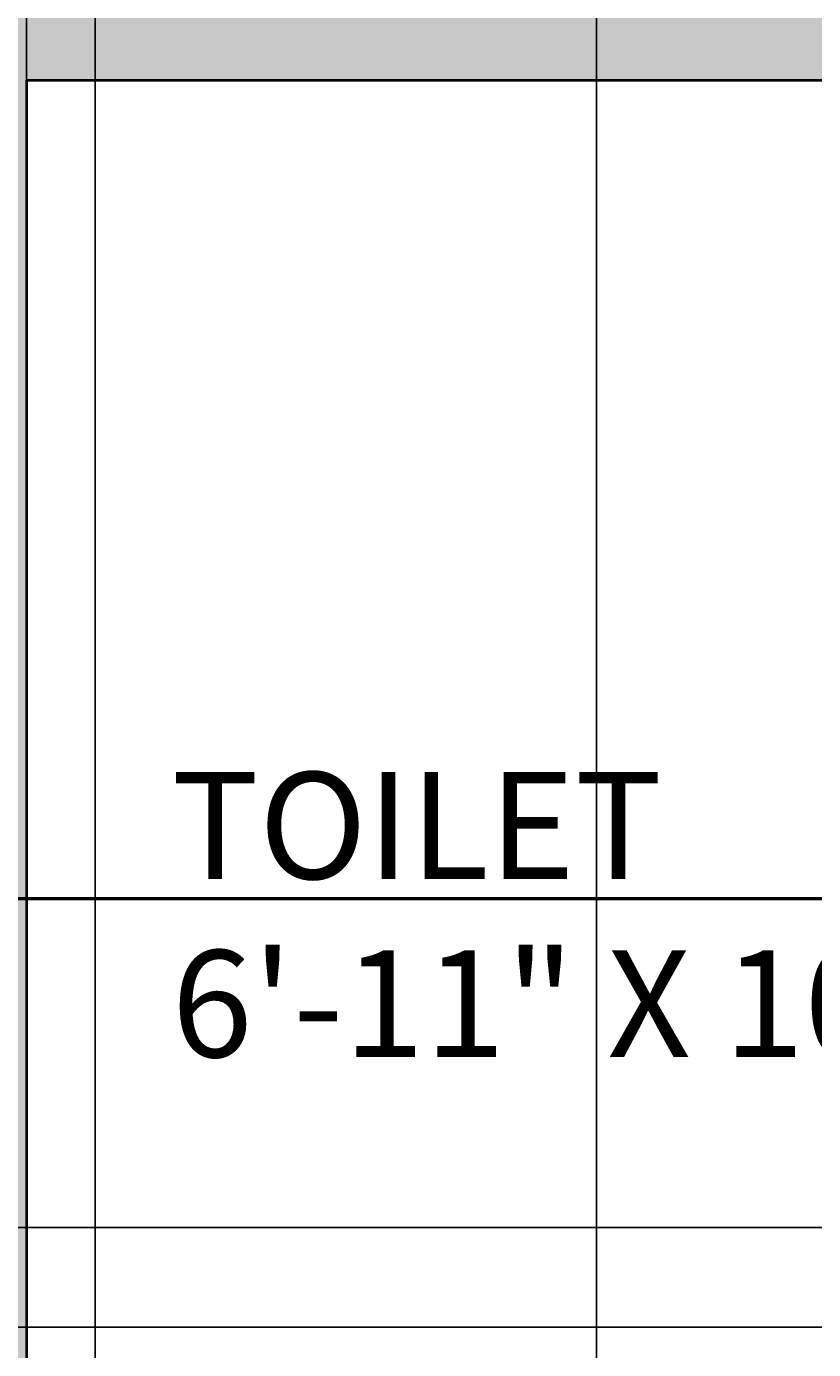
# Model space of a CAD drawing. Units: inches. Extents: x 818 to 1898, y 976 to 2364.
# Tile 45 of 96: x 1623 to 1667, y 1520 to 1594. Entities that reach past the tile are written whole.
import ezdxf

# ---------------------------------------------------------------- set-up
doc = ezdxf.new("R2010")
doc.units = ezdxf.units.IN
doc.header["$LTSCALE"] = 5
doc.header["$MEASUREMENT"] = 0
for name, color, linetype, lineweight in [('A-ANNO-DIMS', 2, 'Continuous', 18), ('A-AREA-IDEN', 7, 'Continuous', 18), ('A-WALL', 7, 'Continuous', 40)]:
    doc.layers.add(name, color=color, linetype=linetype, lineweight=lineweight)
doc.layers.add('A-WALL-PATT', color=251, linetype='Continuous', lineweight=13, true_color=0x636466)
doc.styles.get("Standard").update_dxf_attribs({"font": 'arial.ttf'})
doc.dimstyles.get("Standard").update_dxf_attribs({"dimtxt": 0.18, "dimasz": 0.18, "dimexe": 0.18, "dimexo": 0.0625, "dimgap": 0.09, "dimtad": 0, "dimtih": 1, "dimtoh": 1, "dimdec": 4, "dimzin": 0, "dimdsep": 46, "dimtxsty": 'Standard', "dimcen": 0.09, "dimadec": 0, "dimazin": 0, "dimtfac": 1, "dimtdec": 4, "dimtofl": 0, "dimtmove": 0, "dimatfit": 3, "dimfxl": 1, "dimtolj": 1, "dimtzin": 0, "dimarcsym": 0})

# ---------------------------------------------------------------- blocks, each defined once
blk = doc.blocks.new('*D102')
at = {"layer": 'A-ANNO-DIMS', "color": 0, "lineweight": -2, "ltscale": 5, "transparency": 16777216}
for p, q in [((1565.483, 1071.118), (1565.483, 2363.873)), ((1565.663, 2363.693), (1595.635, 2363.693)), ((1626.395, 2363.693), (1596.423, 2363.693)), ((1626.575, 1071.118), (1626.575, 2363.873))]:
    blk.add_line(p, q, dxfattribs=at)
at = {"layer": 'A-ANNO-DIMS', "color": 0, "ltscale": 5, "transparency": 16777216}
for points in [[(1565.663, 2363.723), (1565.663, 2363.663), (1565.483, 2363.693)], [(1626.395, 2363.723), (1626.395, 2363.663), (1626.575, 2363.693)]]:
    blk.add_solid(points, dxfattribs=at)
at = {"layer": 'Defpoints', "color": 0, "ltscale": 5, "transparency": 16777216}
for p in [(1626.575, 2363.693), (1565.483, 1071.055), (1626.575, 1071.055)]:
    blk.add_point(p, dxfattribs=at)
at = {"layer": 'A-ANNO-DIMS', "color": 0, "ltscale": 5, "transparency": 16777216, "insert": (1596.029, 2363.693), "char_height": 0.18, "attachment_point": 5}
blk.add_mtext('\\A1;61.09', dxfattribs=at)
blk = doc.blocks.new('*D103')
at = {"layer": 'A-ANNO-DIMS', "color": 0, "lineweight": -2, "ltscale": 5, "transparency": 16777216}
for p, q in [((1626.575, 1071.118), (1626.575, 2363.873)), ((1626.755, 2363.693), (1657.699, 2363.693)), ((1689.291, 2363.693), (1658.348, 2363.693)), ((1689.471, 1071.118), (1689.471, 2363.873))]:
    blk.add_line(p, q, dxfattribs=at)
at = {"layer": 'A-ANNO-DIMS', "color": 0, "ltscale": 5, "transparency": 16777216}
for points in [[(1626.755, 2363.723), (1626.755, 2363.663), (1626.575, 2363.693)], [(1689.291, 2363.723), (1689.291, 2363.663), (1689.471, 2363.693)]]:
    blk.add_solid(points, dxfattribs=at)
at = {"layer": 'Defpoints', "color": 0, "ltscale": 5, "transparency": 16777216}
for p in [(1689.471, 2363.693), (1626.575, 1071.055), (1689.471, 1071.055)]:
    blk.add_point(p, dxfattribs=at)
at = {"layer": 'A-ANNO-DIMS', "color": 0, "ltscale": 5, "transparency": 16777216, "insert": (1658.023, 2363.693), "char_height": 0.18, "attachment_point": 5}
blk.add_mtext('\\A1;62.9', dxfattribs=at)
blk = doc.blocks.new('*D117')
at = {"layer": 'A-ANNO-DIMS', "color": 0, "lineweight": -2, "ltscale": 5, "transparency": 16777216}
for p, q in [((1766.29, 1545.183), (818.026, 1545.183)), ((818.206, 1545.003), (818.206, 1501.178)), ((818.206, 1456.989), (818.206, 1500.814)), ((1766.29, 1456.809), (818.026, 1456.809))]:
    blk.add_line(p, q, dxfattribs=at)
at = {"layer": 'A-ANNO-DIMS', "color": 0, "ltscale": 5, "transparency": 16777216}
for points in [[(818.176, 1545.003), (818.236, 1545.003), (818.206, 1545.183)], [(818.176, 1456.989), (818.236, 1456.989), (818.206, 1456.809)]]:
    blk.add_solid(points, dxfattribs=at)
at = {"layer": 'Defpoints', "color": 0, "ltscale": 5, "transparency": 16777216}
for p in [(818.206, 1545.183), (1766.352, 1545.183), (1766.352, 1456.809)]:
    blk.add_point(p, dxfattribs=at)
at = {"layer": 'A-ANNO-DIMS', "color": 0, "ltscale": 5, "transparency": 16777216, "insert": (818.206, 1500.996), "char_height": 0.18, "attachment_point": 5}
blk.add_mtext('\\A1;88.37', dxfattribs=at)
blk = doc.blocks.new('*D118')
at = {"layer": 'A-ANNO-DIMS', "color": 0, "lineweight": -2, "ltscale": 5, "transparency": 16777216}
for p, q in [((1766.29, 1627.505), (818.026, 1627.505)), ((818.206, 1627.325), (818.206, 1586.526)), ((818.206, 1545.363), (818.206, 1586.162)), ((1766.29, 1545.183), (818.026, 1545.183))]:
    blk.add_line(p, q, dxfattribs=at)
at = {"layer": 'A-ANNO-DIMS', "color": 0, "ltscale": 5, "transparency": 16777216}
for points in [[(818.176, 1627.325), (818.236, 1627.325), (818.206, 1627.505)], [(818.176, 1545.363), (818.236, 1545.363), (818.206, 1545.183)]]:
    blk.add_solid(points, dxfattribs=at)
at = {"layer": 'Defpoints', "color": 0, "ltscale": 5, "transparency": 16777216}
for p in [(818.206, 1627.505), (1766.352, 1627.505), (1766.352, 1545.183)]:
    blk.add_point(p, dxfattribs=at)
at = {"layer": 'A-ANNO-DIMS', "color": 0, "ltscale": 5, "transparency": 16777216, "insert": (818.206, 1586.344), "char_height": 0.18, "attachment_point": 5}
blk.add_mtext('\\A1;82.32', dxfattribs=at)
blk = doc.blocks.new('*D170')
at = {"layer": 'A-ANNO-DIMS', "color": 0, "lineweight": -2, "ltscale": 5, "transparency": 16777216}
for p, q in [((1430.788, 1600.078), (1897.916, 1600.078)), ((1897.736, 1599.898), (1897.736, 1550.76)), ((1897.736, 1501.258), (1897.736, 1550.396)), ((1430.788, 1501.078), (1897.916, 1501.078))]:
    blk.add_line(p, q, dxfattribs=at)
at = {"layer": 'A-ANNO-DIMS', "color": 0, "ltscale": 5, "transparency": 16777216}
for points in [[(1897.706, 1599.898), (1897.766, 1599.898), (1897.736, 1600.078)], [(1897.706, 1501.258), (1897.766, 1501.258), (1897.736, 1501.078)]]:
    blk.add_solid(points, dxfattribs=at)
at = {"layer": 'Defpoints', "color": 0, "ltscale": 5, "transparency": 16777216}
for p in [(1430.725, 1600.078), (1897.736, 1600.078), (1430.725, 1501.078)]:
    blk.add_point(p, dxfattribs=at)
at = {"layer": 'A-ANNO-DIMS', "color": 0, "ltscale": 5, "transparency": 16777216, "insert": (1897.736, 1550.578), "char_height": 0.18, "attachment_point": 5}
blk.add_mtext('\\A1;99', dxfattribs=at)
blk = doc.blocks.new('*D173')
at = {"layer": 'A-ANNO-DIMS', "color": 0, "lineweight": -2, "ltscale": 5, "transparency": 16777216}
for p, q in [((1622.725, 1463.141), (1622.725, 2363.873)), ((1622.905, 2363.693), (1638.507, 2363.693)), ((1654.545, 2363.693), (1638.943, 2363.693)), ((1654.725, 1463.141), (1654.725, 2363.873))]:
    blk.add_line(p, q, dxfattribs=at)
at = {"layer": 'A-ANNO-DIMS', "color": 0, "ltscale": 5, "transparency": 16777216}
for points in [[(1622.905, 2363.723), (1622.905, 2363.663), (1622.725, 2363.693)], [(1654.545, 2363.723), (1654.545, 2363.663), (1654.725, 2363.693)]]:
    blk.add_solid(points, dxfattribs=at)
at = {"layer": 'Defpoints', "color": 0, "ltscale": 5, "transparency": 16777216}
for p in [(1654.725, 2363.693), (1622.725, 1463.078), (1654.725, 1463.078)]:
    blk.add_point(p, dxfattribs=at)
at = {"layer": 'A-ANNO-DIMS', "color": 0, "ltscale": 5, "transparency": 16777216, "insert": (1638.725, 2363.693), "char_height": 0.18, "attachment_point": 5}
blk.add_mtext('\\A1;32', dxfattribs=at)
blk = doc.blocks.new('*D180')
at = {"layer": 'A-ANNO-DIMS', "color": 0, "lineweight": -2, "ltscale": 5, "transparency": 16777216}
for p, q in [((1599.725, 1639.516), (1599.725, 975.663)), ((1669.725, 1639.516), (1669.725, 975.663)), ((1599.905, 975.843), (1634.507, 975.843)), ((1669.545, 975.843), (1634.943, 975.843))]:
    blk.add_line(p, q, dxfattribs=at)
at = {"layer": 'A-ANNO-DIMS', "color": 0, "ltscale": 5, "transparency": 16777216}
for points in [[(1599.905, 975.873), (1599.905, 975.813), (1599.725, 975.843)], [(1669.545, 975.873), (1669.545, 975.813), (1669.725, 975.843)]]:
    blk.add_solid(points, dxfattribs=at)
at = {"layer": 'Defpoints', "color": 0, "ltscale": 5, "transparency": 16777216}
for p in [(1599.725, 1639.578), (1669.725, 1639.578), (1669.725, 975.843)]:
    blk.add_point(p, dxfattribs=at)
at = {"layer": 'A-ANNO-DIMS', "color": 0, "ltscale": 5, "transparency": 16777216, "insert": (1634.725, 975.843), "char_height": 0.18, "attachment_point": 5}
blk.add_mtext('\\A1;70', dxfattribs=at)
blk = doc.blocks.new('*D187')
at = {"layer": 'A-ANNO-DIMS', "color": 0, "lineweight": -2, "ltscale": 5, "transparency": 16777216}
for p, q in [((1705.663, 1545.078), (818.026, 1545.078)), ((818.206, 1544.898), (818.206, 1533.259)), ((818.206, 1521.258), (818.206, 1532.898)), ((1705.663, 1521.078), (818.026, 1521.078))]:
    blk.add_line(p, q, dxfattribs=at)
at = {"layer": 'A-ANNO-DIMS', "color": 0, "ltscale": 5, "transparency": 16777216}
for points in [[(818.176, 1544.898), (818.236, 1544.898), (818.206, 1545.078)], [(818.176, 1521.258), (818.236, 1521.258), (818.206, 1521.078)]]:
    blk.add_solid(points, dxfattribs=at)
at = {"layer": 'Defpoints', "color": 0, "ltscale": 5, "transparency": 16777216}
for p in [(818.206, 1545.078), (1705.725, 1545.078), (1705.725, 1521.078)]:
    blk.add_point(p, dxfattribs=at)
at = {"layer": 'A-ANNO-DIMS', "color": 0, "ltscale": 5, "transparency": 16777216, "insert": (818.206, 1533.078), "char_height": 0.18, "attachment_point": 5}
blk.add_mtext('\\A1;24', dxfattribs=at)
blk = doc.blocks.new('*D197')
at = {"layer": 'A-ANNO-DIMS', "color": 0, "lineweight": -2, "ltscale": 5, "transparency": 16777216}
for p, q in [((1457.788, 1526.671), (1897.916, 1526.671)), ((1897.736, 1526.491), (1897.736, 1468.076)), ((1897.736, 1409.298), (1897.736, 1467.713)), ((1457.788, 1409.118), (1897.916, 1409.118))]:
    blk.add_line(p, q, dxfattribs=at)
at = {"layer": 'A-ANNO-DIMS', "color": 0, "ltscale": 5, "transparency": 16777216}
for points in [[(1897.706, 1526.491), (1897.766, 1526.491), (1897.736, 1526.671)], [(1897.706, 1409.298), (1897.766, 1409.298), (1897.736, 1409.118)]]:
    blk.add_solid(points, dxfattribs=at)
at = {"layer": 'Defpoints', "color": 0, "ltscale": 5, "transparency": 16777216}
for p in [(1457.725, 1526.671), (1897.736, 1526.671), (1457.725, 1409.118)]:
    blk.add_point(p, dxfattribs=at)
at = {"layer": 'A-ANNO-DIMS', "color": 0, "ltscale": 5, "transparency": 16777216, "insert": (1897.736, 1467.894), "char_height": 0.18, "attachment_point": 5}
blk.add_mtext('\\A1;117.55', dxfattribs=at)
blk = doc.blocks.new('*D198')
at = {"layer": 'A-ANNO-DIMS', "color": 0, "lineweight": -2, "ltscale": 5, "transparency": 16777216}
for p, q in [((1741.841, 1545.016), (1741.841, 975.663)), ((1430.725, 1346.016), (1430.725, 975.663)), ((1430.905, 975.843), (1585.907, 975.843)), ((1741.661, 975.843), (1586.659, 975.843))]:
    blk.add_line(p, q, dxfattribs=at)
at = {"layer": 'A-ANNO-DIMS', "color": 0, "ltscale": 5, "transparency": 16777216}
for points in [[(1430.905, 975.873), (1430.905, 975.813), (1430.725, 975.843)], [(1741.661, 975.873), (1741.661, 975.813), (1741.841, 975.843)]]:
    blk.add_solid(points, dxfattribs=at)
at = {"layer": 'Defpoints', "color": 0, "ltscale": 5, "transparency": 16777216}
for p in [(1741.841, 1545.078), (1430.725, 1346.078), (1741.841, 975.843)]:
    blk.add_point(p, dxfattribs=at)
at = {"layer": 'A-ANNO-DIMS', "color": 0, "ltscale": 5, "transparency": 16777216, "insert": (1586.283, 975.843), "char_height": 0.18, "attachment_point": 5}
blk.add_mtext('\\A1;311.1', dxfattribs=at)
blk = doc.blocks.new('*D199')
at = {"layer": 'A-ANNO-DIMS', "color": 0, "lineweight": -2, "ltscale": 5, "transparency": 16777216}
for p, q in [((1559.788, 1687.078), (1897.916, 1687.078)), ((1897.736, 1686.898), (1897.736, 1513.154)), ((1897.736, 1339.045), (1897.736, 1512.79)), ((1660.377, 1338.865), (1897.916, 1338.865))]:
    blk.add_line(p, q, dxfattribs=at)
at = {"layer": 'A-ANNO-DIMS', "color": 0, "ltscale": 5, "transparency": 16777216}
for points in [[(1897.706, 1686.898), (1897.766, 1686.898), (1897.736, 1687.078)], [(1897.706, 1339.045), (1897.766, 1339.045), (1897.736, 1338.865)]]:
    blk.add_solid(points, dxfattribs=at)
at = {"layer": 'Defpoints', "color": 0, "ltscale": 5, "transparency": 16777216}
for p in [(1559.725, 1687.078), (1897.736, 1687.078), (1660.314, 1338.865)]:
    blk.add_point(p, dxfattribs=at)
at = {"layer": 'A-ANNO-DIMS', "color": 0, "ltscale": 5, "transparency": 16777216, "insert": (1897.736, 1512.972), "char_height": 0.18, "attachment_point": 5}
blk.add_mtext('\\A1;348.2', dxfattribs=at)
blk = doc.blocks.new('*D214')
at = {"layer": 'A-ANNO-DIMS', "color": 0, "lineweight": -2, "ltscale": 5, "transparency": 16777216}
for p, q in [((1511.725, 1687.016), (1511.725, 975.663)), ((1714.725, 1687.016), (1714.725, 975.663)), ((1511.905, 975.843), (1612.935, 975.843)), ((1714.545, 975.843), (1613.516, 975.843))]:
    blk.add_line(p, q, dxfattribs=at)
at = {"layer": 'A-ANNO-DIMS', "color": 0, "ltscale": 5, "transparency": 16777216}
for points in [[(1511.905, 975.873), (1511.905, 975.813), (1511.725, 975.843)], [(1714.545, 975.873), (1714.545, 975.813), (1714.725, 975.843)]]:
    blk.add_solid(points, dxfattribs=at)
at = {"layer": 'Defpoints', "color": 0, "ltscale": 5, "transparency": 16777216}
for p in [(1511.725, 1687.078), (1714.725, 1687.078), (1714.725, 975.843)]:
    blk.add_point(p, dxfattribs=at)
at = {"layer": 'A-ANNO-DIMS', "color": 0, "ltscale": 5, "transparency": 16777216, "insert": (1613.225, 975.843), "char_height": 0.18, "attachment_point": 5}
blk.add_mtext('\\A1;203', dxfattribs=at)

msp = doc.modelspace()

# ---------------------------------------------------------------- hatches: boundary and pattern name
at = {"layer": 'A-WALL-PATT', "ltscale": 5}
h = msp.add_hatch(color=256, dxfattribs=at)
h.dxf.hatch_style = 1
h.paths.add_polyline_path([(1267.7252, 1928.9218), (1258.7252, 1928.9218), (1258.7252, 1913.6401), (1250.3029, 1913.6401), (1250.3029, 1878.3919), (1258.7252, 1878.3919), (1258.7252, 1862.9652), (1267.7252, 1862.9652)])
h.paths.add_polyline_path([(1267.7252, 1814.9652), (1258.7252, 1814.9652), (1258.7252, 1755.3321), (1267.7252, 1755.3321)])
h.paths.add_polyline_path([(1463.7252, 1696.0782), (1267.7252, 1696.0782), (1267.7252, 1707.3321), (1258.7252, 1707.3321), (1258.7252, 1700.0782), (1251.9333, 1700.0782), (1251.9333, 1687.0782), (1463.7252, 1687.0782)])
h.paths.add_polyline_path([(1714.7251, 1717.3178), (1705.7251, 1717.3178), (1705.7251, 1696.0782), (1599.7251, 1696.0782), (1599.7251, 1790.0782), (1705.7251, 1790.0782), (1705.7251, 1785.6125), (1714.7251, 1785.6125), (1714.7251, 1827.2125), (1705.7251, 1827.2125), (1705.7251, 1802.0782), (1599.7251, 1802.0782), (1599.7251, 1867.0782), (1705.7251, 1867.0782), (1705.7251, 1857.2125), (1714.7251, 1857.2125), (1714.7251, 1930.0316), (1741.8409, 1930.0316), (1741.8409, 1935.0316), (1714.7251, 1935.0316), (1714.7251, 1957.0338), (1741.8409, 1957.0338), (1741.8409, 1962.0338), (1714.7251, 1962.0338), (1705.7251, 1962.0338), (1705.7251, 1948.0782), (1599.7251, 1948.0782), (1599.7251, 1981.0782), (1590.7252, 1981.0782), (1590.7252, 1941.0782), (1620.7252, 1941.0782), (1705.7251, 1941.0782), (1705.7251, 1876.0782), (1599.7251, 1876.0782), (1599.7251, 1911.0782), (1590.7252, 1911.0782), (1590.7252, 1876.0782), (1429.2252, 1876.0782), (1429.2252, 1867.0782), (1511.7251, 1867.0782), (1528.593, 1867.0782), (1595.7252, 1867.0782), (1595.7252, 1773.0782), (1520.7252, 1773.0782), (1520.7252, 1837.5823), (1532.593, 1837.5823), (1532.593, 1867.0782), (1528.593, 1867.0782), (1528.593, 1841.5823), (1511.7251, 1841.5823), (1511.7251, 1744.9714), (1520.7252, 1744.9714), (1520.7252, 1761.0782), (1595.7252, 1761.0782), (1595.7252, 1696.0782), (1520.7252, 1696.0782), (1520.7252, 1716.0454), (1511.7251, 1716.0454), (1511.7251, 1696.0782), (1511.7251, 1687.0782), (1714.7251, 1687.0782)])
h.paths.add_polyline_path([(1714.7251, 2053.0782), (1714.7251, 2081.1881), (1709.7252, 2081.1881), (1709.7252, 2053.0782), (1681.6446, 2053.0782), (1681.6446, 2081.1881), (1676.6446, 2081.1881), (1676.6446, 2053.0782), (1538.5155, 2053.0782), (1538.5155, 2044.0782), (1590.7252, 2044.0782), (1590.7252, 2011.0782), (1599.7251, 2011.0782), (1599.7251, 2044.0782), (1705.7251, 2044.0782), (1705.7251, 2014.5114), (1714.7251, 2014.5114)])
h.paths.add_polyline_path([(1485.1216, 2053.0782), (1422.02, 2053.0782), (1422.02, 2081.1881), (1413.02, 2081.1881), (1413.02, 2053.0782), (1399.6356, 2053.0782), (1399.6356, 2081.1881), (1390.6356, 2081.1881), (1390.6356, 2053.0782), (1388.0315, 2053.0782), (1388.0315, 2044.0782), (1416.2743, 2044.0782), (1485.1216, 2044.0782)])
h.paths.add_polyline_path([(1330.305, 2053.0782), (1258.7252, 2053.0782), (1258.7252, 2019.2871), (1267.7252, 2019.2871), (1267.7252, 2044.0782), (1330.305, 2044.0782)])
h.paths.add_polyline_path([(1258.7252, 2053.0782), (1214.6577, 2053.0782), (1214.6577, 2044.0782), (1258.7252, 2044.0782)])
h.paths.add_polyline_path([(1214.6577, 2053.0782), (1180.349, 2053.0782), (1180.349, 2044.0782), (1214.6577, 2044.0782)])
h.paths.add_polyline_path([(1714.7251, 1639.5782), (1741.8409, 1639.5782), (1741.8409, 1643.5782), (1714.7251, 1643.5782), (1714.7251, 1649.9029), (1705.7251, 1649.9029), (1705.7251, 1600.0782), (1477.7252, 1600.0782), (1477.7252, 1591.0782), (1520.7252, 1591.0782), (1616.7252, 1591.0782), (1616.7252, 1416.6857), (1622.7251, 1416.6857), (1622.7251, 1463.0782), (1624.7252, 1463.0782), (1624.7252, 1467.0782), (1622.7251, 1467.0782), (1622.7251, 1591.0782), (1705.7251, 1591.0782), (1705.7251, 1545.0782), (1714.7251, 1545.0782), (1741.8409, 1545.0782), (1741.8409, 1549.0782), (1714.7251, 1549.0782), (1714.7251, 1593.9175), (1737.8409, 1593.9175), (1737.8409, 1597.9175), (1714.7251, 1597.9175)])
h.paths.add_polyline_path([(1674.9024, 2060.7419), (1714.7045, 2060.7419), (1714.7045, 2073.1061), (1674.9024, 2073.1061)], flags=25)
h.paths.add_polyline_path([(1394.5468, 2061.6618), (1422.2344, 2061.6618), (1422.2344, 2074.0261), (1394.5468, 2074.0261)], flags=24)

# ---------------------------------------------------------------- linework, layer by layer
at = {"layer": 'A-WALL'}
for q in [(1622.7251, 1467.0782), (1705.7251, 1591.0782)]:
    msp.add_line((1622.7251, 1591.0782), q, dxfattribs=at)

# ---------------------------------------------------------------- texts
at = {"layer": 'A-AREA-IDEN', "ltscale": 5, "insert": (1630.8716, 1552.2375), "char_height": 6, "attachment_point": 1}
msp.add_mtext_dynamic_manual_height_columns('TOILET\\P6\'-11" X 10\'-4"', width=118.992422, gutter_width=1, heights=[0], dxfattribs=at)

# ---------------------------------------------------------------- dimensions: what is measured, and where the dimension line sits
at = {"layer": 'A-ANNO-DIMS', "ltscale": 5}
for base, p1, p2, override, picture, middle in [((1626.5748, 2363.6929), (1565.4835, 1071.0552), (1626.5748, 1071.0552), {"dimdec": 2, "dimlfac": 1, "dimrnd": 0, "dimzin": 0, "dimdsep": 46, "dimlunit": 2}, '*D102', (1596.0291, 2363.6929)), ((1654.7251, 2363.6929), (1622.7251, 1463.0782), (1654.7251, 1463.0782), {"dimdec": 0, "dimlfac": 1, "dimrnd": 0, "dimzin": 0, "dimdsep": 46, "dimlunit": 2}, '*D173', (1638.7251, 2363.6929)), ((1689.4714, 2363.6929), (1626.5748, 1071.0552), (1689.4714, 1071.0552), {"dimdec": 1, "dimlfac": 1, "dimrnd": 0, "dimzin": 0, "dimdsep": 46, "dimlunit": 2}, '*D103', (1658.0231, 2363.6929)), ((1714.7251, 975.8433), (1511.7251, 1687.0782), (1714.7251, 1687.0782), {"dimdec": 0, "dimlfac": 1, "dimrnd": 0, "dimzin": 0, "dimdsep": 46, "dimlunit": 2}, '*D214', (1613.2251, 975.8433)), ((1669.7251, 975.8433), (1599.7251, 1639.5782), (1669.7251, 1639.5782), {"dimdec": 0, "dimlfac": 1, "dimrnd": 0, "dimzin": 0, "dimdsep": 46, "dimlunit": 2}, '*D180', (1634.7251, 975.8433)), ((1741.8409, 975.8433), (1430.7251, 1346.0782), (1741.8409, 1545.0782), {"dimdec": 1, "dimlfac": 1, "dimrnd": 0, "dimzin": 0, "dimdsep": 46, "dimlunit": 2}, '*D198', (1586.283, 975.8433))]:
    dim = msp.add_linear_dim(base=base, p1=p1, p2=p2, dimstyle='Standard', override=override, dxfattribs=at)
    dim.commit()
    dim.dimension.update_dxf_attribs({"geometry": picture, "text_midpoint": middle})
for base, p1, p2, override, picture, middle in [((1897.736, 1687.0782), (1660.3141, 1338.8654), (1559.7251, 1687.0782), {"dimdec": 1, "dimlfac": 1, "dimrnd": 0, "dimzin": 0, "dimdsep": 46, "dimlunit": 2}, '*D199', (1897.736, 1512.9718)), ((818.2059, 1627.5052), (1766.3524, 1545.1827), (1766.3524, 1627.5052), {"dimdec": 2, "dimlfac": 1, "dimrnd": 0, "dimzin": 0, "dimdsep": 46, "dimlunit": 2}, '*D118', (818.2059, 1586.3439)), ((1897.736, 1600.0782), (1430.7251, 1501.0782), (1430.7251, 1600.0782), {"dimdec": 0, "dimlfac": 1, "dimrnd": 0, "dimzin": 0, "dimdsep": 46, "dimlunit": 2}, '*D170', (1897.736, 1550.5782)), ((818.2059, 1545.1827), (1766.3524, 1456.8088), (1766.3524, 1545.1827), {"dimdec": 2, "dimlfac": 1, "dimrnd": 0, "dimzin": 0, "dimdsep": 46, "dimlunit": 2}, '*D117', (818.2059, 1500.9957)), ((818.2059, 1545.0782), (1705.7251, 1521.0782), (1705.7251, 1545.0782), {"dimdec": 0, "dimlfac": 1, "dimrnd": 0, "dimzin": 0, "dimdsep": 46, "dimlunit": 2}, '*D187', (818.2059, 1533.0782)), ((1897.736, 1526.6712), (1457.7251, 1409.1177), (1457.7251, 1526.6712), {"dimdec": 2, "dimlfac": 1, "dimrnd": 0, "dimzin": 0, "dimdsep": 46, "dimlunit": 2}, '*D197', (1897.736, 1467.8945))]:
    dim = msp.add_linear_dim(base=base, p1=p1, p2=p2, angle=90, dimstyle='Standard', override=override, dxfattribs=at)
    dim.commit()
    dim.dimension.update_dxf_attribs({"geometry": picture, "text_midpoint": middle})

doc.saveas('drawing.dxf')
